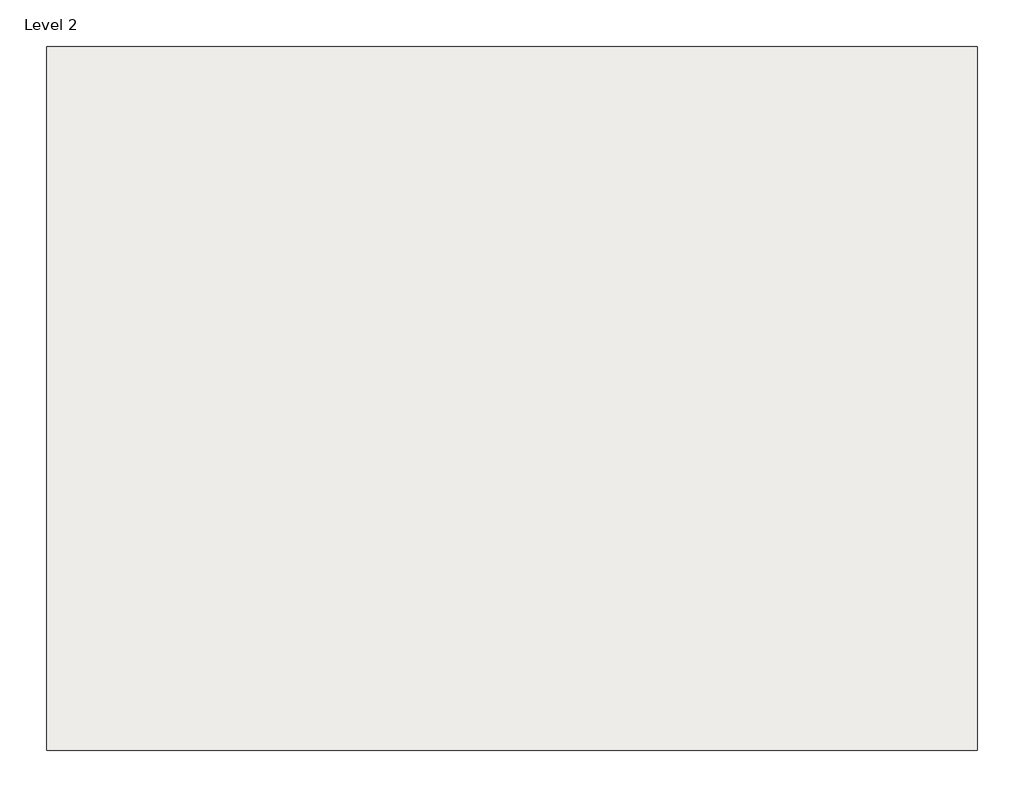
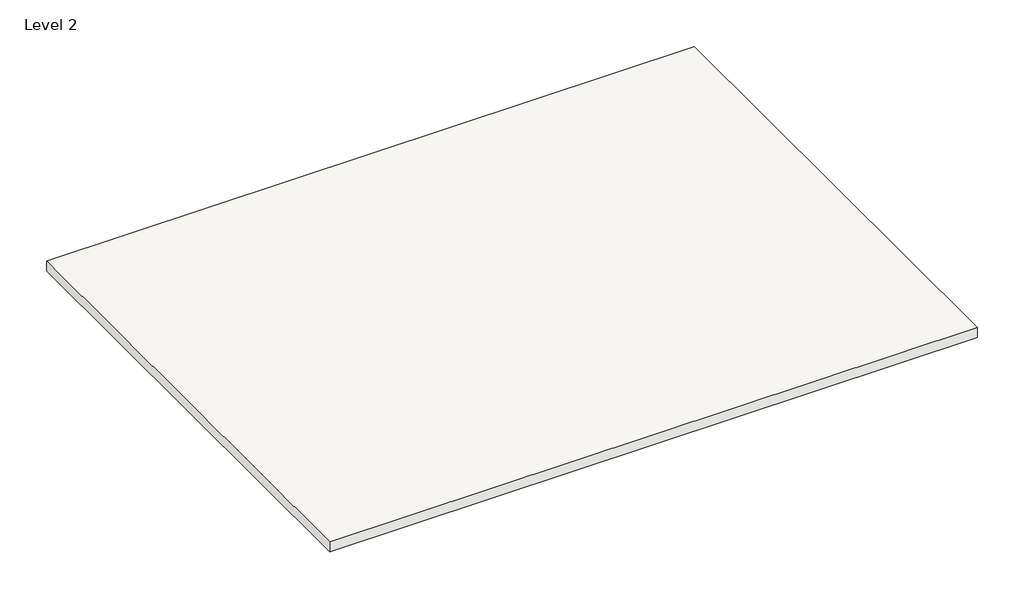
# One storey: 1 roof.
"""IFC4 building model written with IfcOpenShell, lengths in millimetres."""

from ifc_helpers import new_model, si_unit, frame, origin, place, context, project, spatial, polyline, outline, extrude, element, save

model = new_model("IFC4")

# Units and contexts
model_context = context("Model", 3, world=origin())
ifc_project = project(units=[si_unit("LENGTHUNIT", "METRE", prefix="MILLI")], contexts=[model_context])

# Site, building, storey
site = spatial("IfcSite", under=ifc_project)
building = spatial("IfcBuilding", under=site)
storey = spatial("IfcBuildingStorey", under=building, Name="Level 2", Elevation=3048.0)

# Roof
placement = place(None, origin())
element("IfcRoof", 1, ObjectType="Wood Rafter 8\" - Asphalt Shingle - Insulated", at=placement, inside=storey, context=model_context, shape_type="SweptSolid", body=[
    extrude(outline(polyline([(-10781.3447551, 3944.0549175), (-10781.3447551, 13570.6549175), (1944.0552449, 13570.6549175), (1944.0552449, 3944.0549175), (-10781.3447551, 3944.0549175)])), frame((0.0, 0.0, 3048.0), z_axis=(0.0, 0.0, 1.0), x_axis=(1.0, 0.0, 0.0)), (0.0, 0.0, 1.0), 212.725),
])

save(model, "model.ifc")

# Revit data of these elements
# Type "Wood Rafter 8\" - Asphalt Shingle - Insulated"
#   Assembly Code = "B1020"
#   Layers, outside or top first: 0' - 0 1/4" "Asphalt Shingle" (function 4); 0' - 0 5/8" "Plywood, Sheathing" (function 2); 0' - 7 1/2" "Structure, Wood Joist/Rafter Layer, Batt Insulation" (function 1)
# Element 1 (IfcRoof, "Wood Rafter 8\" - Asphalt Shingle - Insulated")
#   built-in parameter 1001705 = 10.6979 (stored number, unit not read)
#   built-in parameter 1001710 = 33615
#   Phase Created = New Construction
#   Materials on its faces: "Structure, Wood Joist/Rafter Layer, Batt Insulation", "Asphalt Shingle"
# Materials
#   "Asphalt Shingle": class "Generic", colour RGB 155 155 155, transparency 0, Description = "Asphalt roofing shingle", Cost = 0
#   "Plywood, Sheathing": class "Wood", colour RGB 212 179 113, transparency 0, Description = "Plywood, sheathing grade", Cost = 0
#   "Structure, Wood Joist/Rafter Layer, Batt Insulation": class "Wood", colour RGB 127 127 127, transparency 0, Description = "Wood framing, insulated", Cost = 0
